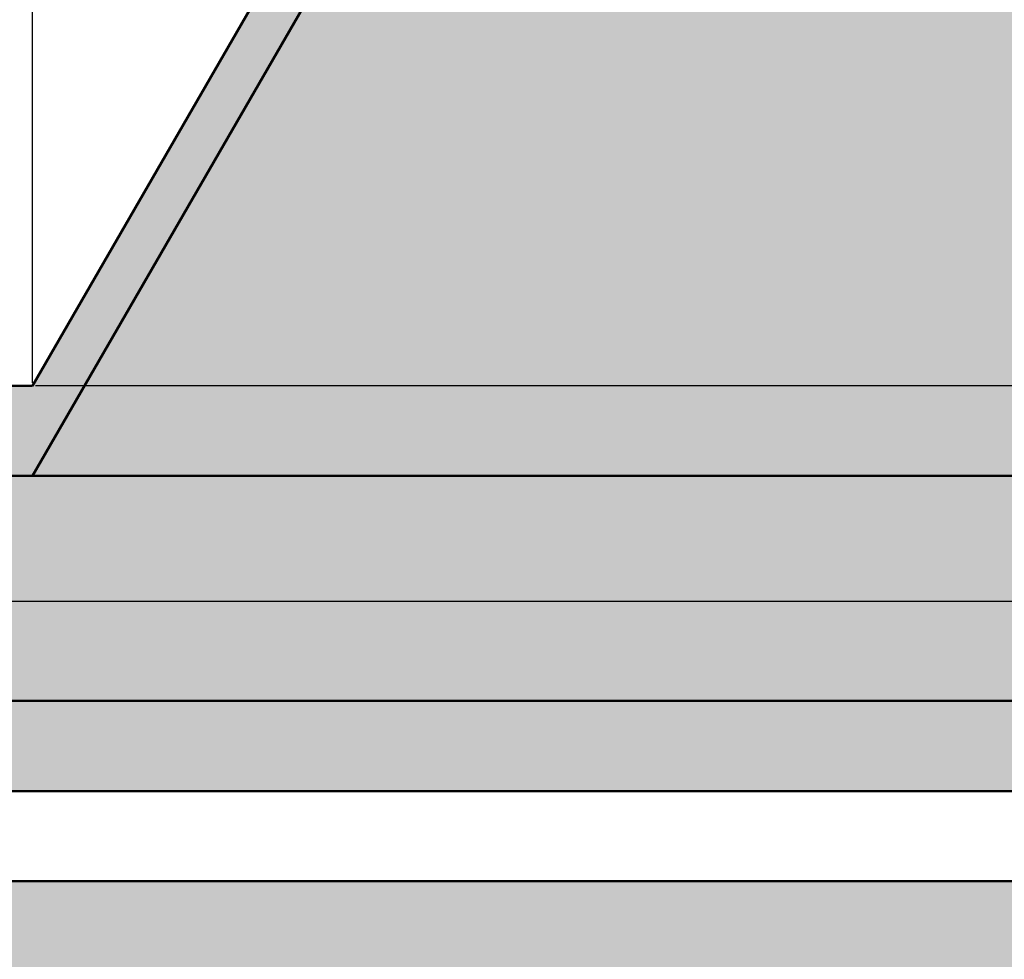
# Model space of a CAD drawing. Units: inches. Extents: x -12 to 334, y -10 to 186.
# Tile 39 of 77: x 106 to 128, y 90 to 111. Entities that reach past the tile are written whole.
import ezdxf
from ezdxf import colors
from ezdxf.entities.mleader import LeaderData, LeaderLine
from ezdxf.math import Vec2, Vec3

# ---------------------------------------------------------------- set-up
doc = ezdxf.new("R2010")
doc.units = ezdxf.units.IN
doc.header["$MEASUREMENT"] = 0
for name, color, linetype, lineweight in [('M-ANNO-TEXT', 3, 'Continuous', 25), ('M-DIMS', 2, 'Continuous', 18), ('M-EQPM', 7, 'Continuous', 50), ('M-EQPM-PATT', 8, 'Continuous', 18)]:
    doc.layers.add(name, color=color, linetype=linetype, lineweight=lineweight)
doc.styles.get("Standard").update_dxf_attribs({"font": 'arial.ttf'})
doc.dimstyles.get("Standard").update_dxf_attribs({"dimtxt": 0.18, "dimasz": 0.18, "dimexe": 0.18, "dimexo": 0.0625, "dimgap": 0.09, "dimtad": 0, "dimtih": 1, "dimtoh": 1, "dimdec": 4, "dimzin": 0, "dimdsep": 46, "dimtxsty": 'Standard', "dimcen": 0.09, "dimadec": 0, "dimazin": 0, "dimtfac": 1, "dimtdec": 4, "dimtofl": 0, "dimtmove": 0, "dimatfit": 3, "dimfxl": 1, "dimtolj": 1, "dimtzin": 0, "dimarcsym": 0})

# ---------------------------------------------------------------- blocks, each defined once
blk = doc.blocks.new('*D1')
at = {"layer": 'Defpoints', "color": 0, "transparency": 16777216}
for p in [(281.426, 91.899), (3.376, 80.692), (281.426, 14.304)]:
    blk.add_point(p, dxfattribs=at)
at = {"layer": 'M-DIMS', "color": 0, "lineweight": -2, "transparency": 16777216}
for p, q in [((281.426, 91.836), (281.426, 14.124)), ((3.376, 80.629), (3.376, 14.124)), ((3.556, 14.304), (141.935, 14.304)), ((281.246, 14.304), (142.867, 14.304))]:
    blk.add_line(p, q, dxfattribs=at)
at = {"layer": 'M-DIMS', "color": 0, "transparency": 16777216}
for points in [[(3.556, 14.334), (3.556, 14.274), (3.376, 14.304)], [(281.246, 14.334), (281.246, 14.274), (281.426, 14.304)]]:
    blk.add_solid(points, dxfattribs=at)
at = {"layer": 'M-DIMS', "color": 0, "transparency": 16777216, "insert": (142.401, 14.304), "char_height": 0.18, "attachment_point": 5}
blk.add_mtext('\\A1;278.05', dxfattribs=at)
blk = doc.blocks.new('*D15')
at = {"layer": 'Defpoints', "color": 0, "transparency": 16777216}
for p in [(106.177, 169.385), (86.888, 109.058), (106.177, 102.896)]:
    blk.add_point(p, dxfattribs=at)
at = {"layer": 'M-DIMS', "color": 0, "lineweight": -2, "transparency": 16777216}
for p, q in [((86.888, 109.121), (86.888, 169.565)), ((87.068, 169.385), (96.147, 169.385)), ((105.997, 169.385), (96.918, 169.385)), ((106.177, 102.958), (106.177, 169.565))]:
    blk.add_line(p, q, dxfattribs=at)
at = {"layer": 'M-DIMS', "color": 0, "transparency": 16777216}
for points in [[(87.068, 169.415), (87.068, 169.355), (86.888, 169.385)], [(105.997, 169.415), (105.997, 169.355), (106.177, 169.385)]]:
    blk.add_solid(points, dxfattribs=at)
at = {"layer": 'M-DIMS', "color": 0, "transparency": 16777216, "insert": (96.532, 169.385), "char_height": 0.18, "attachment_point": 5}
blk.add_mtext('\\A1;19.29', dxfattribs=at)
blk = doc.blocks.new('*D16')
at = {"layer": 'Defpoints', "color": 0, "transparency": 16777216}
for p in [(126.379, 169.385), (126.379, 137.887), (106.177, 102.896)]:
    blk.add_point(p, dxfattribs=at)
at = {"layer": 'M-DIMS', "color": 0, "lineweight": -2, "transparency": 16777216}
for p, q in [((106.177, 102.958), (106.177, 169.565)), ((106.357, 169.385), (115.814, 169.385)), ((126.199, 169.385), (116.742, 169.385)), ((126.379, 137.95), (126.379, 169.565))]:
    blk.add_line(p, q, dxfattribs=at)
at = {"layer": 'M-DIMS', "color": 0, "transparency": 16777216}
for points in [[(106.357, 169.415), (106.357, 169.355), (106.177, 169.385)], [(126.199, 169.415), (126.199, 169.355), (126.379, 169.385)]]:
    blk.add_solid(points, dxfattribs=at)
at = {"layer": 'M-DIMS', "color": 0, "transparency": 16777216, "insert": (116.278, 169.385), "char_height": 0.18, "attachment_point": 5}
blk.add_mtext('\\A1;20.202', dxfattribs=at)
blk = doc.blocks.new('*D17')
at = {"layer": 'Defpoints', "color": 0, "transparency": 16777216}
for p in [(106.177, 102.896), (105.892, 56.321), (295.976, 56.321)]:
    blk.add_point(p, dxfattribs=at)
at = {"layer": 'M-DIMS', "color": 0, "lineweight": -2, "transparency": 16777216}
for p, q in [((106.24, 102.896), (296.156, 102.896)), ((295.976, 102.716), (295.976, 79.79)), ((295.976, 56.501), (295.976, 79.426)), ((105.954, 56.321), (296.156, 56.321))]:
    blk.add_line(p, q, dxfattribs=at)
at = {"layer": 'M-DIMS', "color": 0, "transparency": 16777216}
for points in [[(295.946, 102.716), (296.006, 102.716), (295.976, 102.896)], [(295.946, 56.501), (296.006, 56.501), (295.976, 56.321)]]:
    blk.add_solid(points, dxfattribs=at)
at = {"layer": 'M-DIMS', "color": 0, "transparency": 16777216, "insert": (295.976, 79.608), "char_height": 0.18, "attachment_point": 5}
blk.add_mtext('\\A1;46.575', dxfattribs=at)
blk = doc.blocks.new('*D35')
at = {"layer": 'Defpoints', "color": 0, "transparency": 16777216}
for p in [(216.428, 98.108), (-11.174, 61.105), (216.428, 61.105)]:
    blk.add_point(p, dxfattribs=at)
at = {"layer": 'M-DIMS', "color": 0, "lineweight": -2, "transparency": 16777216}
for p, q in [((216.365, 98.108), (-11.354, 98.108)), ((-11.174, 97.928), (-11.174, 79.788)), ((-11.174, 61.285), (-11.174, 79.424)), ((216.365, 61.105), (-11.354, 61.105))]:
    blk.add_line(p, q, dxfattribs=at)
at = {"layer": 'M-DIMS', "color": 0, "transparency": 16777216}
for points in [[(-11.204, 97.928), (-11.144, 97.928), (-11.174, 98.108)], [(-11.204, 61.285), (-11.144, 61.285), (-11.174, 61.105)]]:
    blk.add_solid(points, dxfattribs=at)
at = {"layer": 'M-DIMS', "color": 0, "transparency": 16777216, "insert": (-11.174, 79.606), "char_height": 0.18, "attachment_point": 5}
blk.add_mtext('\\A1;37', dxfattribs=at)

msp = doc.modelspace()

# ---------------------------------------------------------------- hatches: boundary and pattern name
at = {"layer": 'M-EQPM-PATT', "transparency": 33554556}
h = msp.add_hatch(color=256, dxfattribs=at)
h.set_gradient(color1=(248, 206, 179), color2=(248, 206, 179), tint=1)
h.paths.add_polyline_path([(179.7818, 136.8871), (126.9567, 136.8871), (106.1771, 100.8958), (171.5458, 100.8958)])
h.paths.add_polyline_path([(268.3808, 136.9435), (214.0166, 136.9435), (214.0166, 154.8345), (196.3421, 154.8345), (196.3421, 136.8871), (179.7818, 136.8871), (171.5458, 100.8958), (231.7758, 100.8958, -0.4142136), (251.9801, 80.6915), (279.7263, 80.6915, 0.1631825)])
at = {"layer": 'M-EQPM-PATT'}
h = msp.add_hatch(color=256, dxfattribs=at)
h.set_gradient(color1=(99, 100, 102), color2=(99, 100, 102), tint=1)
h.paths.add_polyline_path([(126.9567, 136.8871), (179.7818, 136.8871), (180.0106, 137.8871), (126.3793, 137.8871), (106.1771, 102.8958), (86.8879, 102.8958), (86.8879, 109.0583), (84.7229, 109.0583), (84.7229, 100.8958), (106.1771, 100.8958)])
h.paths.add_polyline_path([(196.3421, 152.8345), (195.3421, 152.8345), (195.3421, 137.8871), (180.0106, 137.8871), (179.7818, 136.8871), (196.3421, 136.8871)])
h.paths.add_polyline_path([(215.0166, 152.8345), (214.0166, 152.8345), (214.0166, 136.9435), (268.3808, 136.9435, -0.2673785), (268.3808, 46.8541), (249.3759, 46.8541), (249.8485, 45.8541), (269.3808, 45.8541, 0.2615891), (269.3808, 137.9435), (215.0166, 137.9435)])
h = msp.add_hatch(color=256, dxfattribs=at)
h.set_gradient(color1=(205, 32, 39), color2=(205, 32, 39), tint=1)
h.paths.add_polyline_path([(64.5, 80.754), (64.5, 89.8963), (226.6083, 89.8963, -1), (226.6083, 69.6117), (64.5, 69.6117), (64.5, 78.754), (4.4744, 78.754, 0.384914), (23.5807, 61.4872), (37.1002, 61.4872), (37.1002, 33.6752), (53.1002, 33.6752), (53.1002, 61.4872), (64.5, 61.4872), (64.5, 63.6117), (226.6083, 63.6117, 1), (226.6083, 95.8963), (64.5, 95.8963), (64.5, 99.8958), (53.1002, 99.8958), (53.1002, 127.7078), (37.1002, 127.7078), (37.1002, 99.8958), (23.5807, 99.8958, 0.4132606), (4.3766, 80.754)])
h.paths.add_polyline_path([(64.5, 91.8963), (64.5, 93.8963), (226.6083, 93.8963, -1), (226.6083, 65.6117), (64.5, 65.6117), (64.5, 67.6117), (226.6083, 67.6117, 1), (226.6083, 91.8963)], flags=16)
h = msp.add_hatch(color=256, dxfattribs=at)
h.set_gradient(color1=(94, 103, 175), color2=(94, 103, 175), tint=1)
h.paths.add_polyline_path([(129.093, 89.8963), (86.8879, 89.8963), (86.8879, 69.6117), (129.093, 69.6117)], flags=17)
h.paths.add_polyline_path([(170.9079, 89.8963), (130.8573, 89.8963), (130.8573, 69.6117), (170.9079, 69.6117)], flags=17)
h.paths.add_polyline_path([(216.4278, 89.8963), (172.6722, 89.8963), (172.6722, 69.6117), (216.4278, 69.6117)], flags=17)
h.paths.add_polyline_path([(245.9354, 82.6969), (247.9354, 82.6969), (247.9354, 46.8541), (268.3808, 46.8541, 0.0998398), (279.7263, 80.6915), (251.9801, 80.6915, 0.4142136), (231.7758, 100.8958), (84.7229, 100.8958), (84.7229, 109.0583), (83.7229, 109.0583), (83.7229, 95.8963), (129.093, 95.8963), (129.093, 98.1081), (130.8573, 98.1081), (130.8573, 95.8963), (170.9079, 95.8963), (170.9079, 98.1081), (172.6722, 98.1081), (172.6722, 95.8963), (216.4278, 95.8963), (216.4278, 98.1081), (218.1922, 98.1081), (218.1922, 95.8963), (226.6083, 95.8963, -1), (226.6083, 63.6117), (218.1922, 63.6117), (218.1922, 61.1045), (216.4278, 61.1045), (216.4278, 63.6117), (172.6722, 63.6117), (172.6722, 61.1045), (170.9079, 61.1045), (170.9079, 63.6117), (130.8573, 63.6117), (130.8573, 61.1045), (129.093, 61.1045), (129.093, 63.6117), (87.8879, 63.6117), (87.8879, 56.3205), (105.8919, 56.3205), (105.8919, 28.8541), (115.8919, 28.8541), (115.8919, 46.8541), (222.5761, 46.8541), (222.5761, 30.8541), (232.5761, 30.8541), (232.5761, 46.8541), (245.9354, 46.8541)])
h.paths.add_polyline_path([(86.8879, 89.8963), (75.9244, 89.8963), (75.9244, 69.6117), (86.8879, 69.6117)])
h.paths.add_polyline_path([(83.7229, 109.0583), (75.9244, 109.0583), (75.9244, 95.8963), (83.7229, 95.8963)])
h.paths.add_polyline_path([(226.6083, 89.8963), (218.1922, 89.8963), (218.1922, 69.6117), (226.6083, 69.6117, 1)], flags=17)
h = msp.add_hatch(color=256, dxfattribs=at)
h.set_gradient(color1=(0, 0, 255), color2=(0, 0, 255), tint=1)
h.paths.add_polyline_path([(84.7229, 100.8958), (84.7229, 109.0583), (83.7229, 109.0583), (83.7229, 95.8963), (129.093, 95.8963), (129.093, 98.1081), (130.8573, 98.1081), (130.8573, 95.8963), (170.9079, 95.8963), (170.9079, 98.1081), (172.6722, 98.1081), (172.6722, 95.8963), (216.4278, 95.8963), (216.4278, 98.1081), (218.1922, 98.1081), (218.1922, 95.8963), (226.6083, 95.8963, -1), (226.6083, 63.6117), (218.1922, 63.6117), (218.1922, 61.1045), (216.4278, 61.1045), (216.4278, 63.6117), (172.6722, 63.6117), (172.6722, 61.1045), (170.9079, 61.1045), (170.9079, 63.6117), (130.8573, 63.6117), (130.8573, 61.1045), (129.093, 61.1045), (129.093, 63.6117), (87.8879, 63.6117), (87.8879, 56.3205), (105.8919, 56.3205), (105.8919, 28.8541), (115.8919, 28.8541), (115.8919, 46.8541), (222.5761, 46.8541), (222.5761, 30.8541), (232.5761, 30.8541), (232.5761, 46.8541), (245.9354, 46.8541), (245.9354, 82.6969), (247.9354, 82.6969), (247.9354, 46.8541), (268.3808, 46.8541, 0.0998398), (279.7263, 80.6915), (251.9801, 80.6915, 0.4142136), (231.7758, 100.8958)])

# ---------------------------------------------------------------- linework, layer by layer
at = {"layer": 'M-EQPM'}
for points in [[(106.1771, 100.8958), (126.9567, 136.8871), (196.3421, 136.8871), (196.3421, 154.8345)], [(106.1771, 102.8958), (126.3793, 137.8871), (195.3421, 137.8871), (195.3421, 152.8345)], [(86.8879, 102.8958), (106.1771, 102.8958)], [(84.7229, 100.8958), (231.7758, 100.8958)]]:
    msp.add_lwpolyline(points, dxfattribs=at)
for points in [[(64.5, 63.6117), (226.6083, 63.6117, 1), (226.6083, 95.8963), (64.5, 95.8963)], [(64.5, 65.6117), (226.6083, 65.6117, 1), (226.6083, 93.8963), (64.5, 93.8963)], [(64.5, 67.6117), (226.6083, 67.6117, 1), (226.6083, 91.8963), (64.5, 91.8963)]]:
    msp.add_lwpolyline(points, format="xyb", dxfattribs=at)

# ---------------------------------------------------------------- dimensions: what is measured, and where the dimension line sits
at = {"layer": 'M-DIMS'}
for base, p1, p2, override, picture, middle in [((106.1771, 169.3845), (86.8879, 109.0583), (106.1771, 102.8958), {"dimdec": 2, "dimlfac": 1, "dimrnd": 0, "dimzin": 0, "dimdsep": 46, "dimlunit": 2}, '*D15', (96.5325, 169.3845)), ((126.3793, 169.3845), (106.1771, 102.8958), (126.3793, 137.8871), {"dimdec": 3, "dimlfac": 1, "dimrnd": 0, "dimzin": 0, "dimdsep": 46, "dimlunit": 2}, '*D16', (116.2782, 169.3845)), ((281.4256, 14.3041), (3.3765, 80.6915), (281.4256, 91.8988), {"dimdec": 2, "dimlfac": 1, "dimrnd": 0, "dimzin": 0, "dimdsep": 46, "dimlunit": 2}, '*D1', (142.401, 14.3041))]:
    dim = msp.add_linear_dim(base=base, p1=p1, p2=p2, dimstyle='Standard', override=override, dxfattribs=at)
    dim.commit()
    dim.dimension.update_dxf_attribs({"geometry": picture, "text_midpoint": middle})
for base, p1, p2, override, picture, middle in [((295.9756, 56.3205), (106.1771, 102.8958), (105.8919, 56.3205), {"dimdec": 3, "dimlfac": 1, "dimrnd": 0, "dimzin": 0, "dimdsep": 46, "dimlunit": 2}, '*D17', (295.9756, 79.6082)), ((-11.1736, 61.1045), (216.4278, 98.1081), (216.4278, 61.1045), {"dimdec": 0, "dimlfac": 1, "dimrnd": 0, "dimzin": 0, "dimdsep": 46, "dimlunit": 2}, '*D35', (-11.1735, 79.6063))]:
    dim = msp.add_linear_dim(base=base, p1=p1, p2=p2, angle=90, dimstyle='Standard', override=override, dxfattribs=at)
    dim.commit()
    dim.dimension.update_dxf_attribs({"geometry": picture, "text_midpoint": middle})

# ---------------------------------------------------------------- leaders
at = {"layer": 'M-ANNO-TEXT'}
ml = msp.add_multileader_mtext('Standard', dxfattribs=at)
ml.set_content('Tube plate', color=256)
ml.set_leader_properties()
ml.build(insert=Vec2(0, 0))
ml.multileader.update_dxf_attribs({"dogleg_length": 0.36, "arrow_head_size": 0.7})
ctx = ml.context
ctx.base_point, ctx.arrow_head_size, ctx.landing_gap_size, ctx.plane_origin = Vec3(95.9742, 157.4218), 0.7, 0.09, Vec3(31.4743, 171.7024)
notes = []
notes.append((ctx, [(0, (1, 1, 0), (78.5354, 157.4218), (1, 0), 17.4388, [(0, [(75.9244, 109.0583)], 0, [])])]))
ctx.mtext.insert, ctx.mtext.flow_direction = Vec3(96.0642, 159.9771), 5
for ctx, leaders in notes:
    for number, flags, end, landing, length, lines in leaders:
        leader = LeaderData()
        leader.index, (leader.has_last_leader_line, leader.has_dogleg_vector, leader.attachment_direction) = number, flags
        leader.last_leader_point, leader.dogleg_vector, leader.dogleg_length = Vec3(end), Vec3(landing), length
        for number, points, colour, breaks in lines:
            line = LeaderLine()
            line.index, line.vertices, line.color, line.breaks = number, Vec3.list(points), colors.encode_raw_color(colour), breaks
            leader.lines.append(line)
        ctx.leaders.append(leader)

doc.saveas('drawing.dxf')
